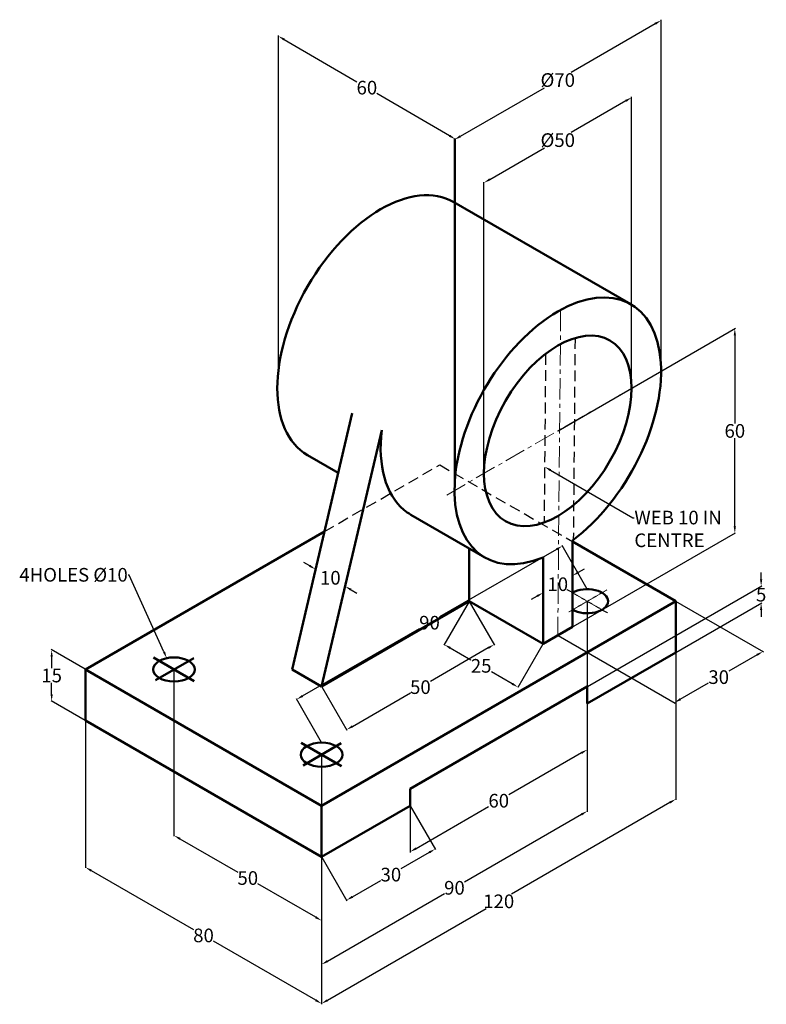
# Model space of a CAD drawing. Units: millimetres. Extents: x -58 to 161, y -39 to 250.
import ezdxf
from ezdxf import colors
from ezdxf.entities.mleader import LeaderData, LeaderLine
from ezdxf.math import Vec2, Vec3

# ---------------------------------------------------------------- set-up
doc = ezdxf.new("R2010")
doc.units = ezdxf.units.MM
doc.header["$MEASUREMENT"] = 0
doc.linetypes.add('CENTER', pattern=[2, 1.25, -0.25, 0.25, -0.25])
doc.linetypes.add('HIDDEN', pattern=[9.525, 6.35, -3.175])
for name, color, linetype, lineweight in [('M-CNTR', 1, 'CENTER', 18), ('M-DIMS', 2, 'Continuous', 25), ('M-HIDN', 3, 'HIDDEN', 25), ('M-OUTL', 7, 'Continuous', 50)]:
    doc.layers.add(name, color=color, linetype=linetype, lineweight=lineweight)
doc.styles.get("Standard").update_dxf_attribs({"font": 'arial.ttf'})
doc.dimstyles.get("Standard").update_dxf_attribs({"dimtxt": 4, "dimasz": 2, "dimexe": 0.18, "dimexo": 0.0625, "dimgap": 0.09, "dimtad": 0, "dimtih": 1, "dimtoh": 1, "dimdec": 0, "dimzin": 0, "dimdsep": 46, "dimtxsty": 'Standard', "dimcen": 0.09, "dimadec": 0, "dimazin": 0, "dimtfac": 1, "dimtdec": 0, "dimtofl": 0, "dimtmove": 0, "dimatfit": 3, "dimfxl": 1, "dimtolj": 1, "dimtzin": 0, "dimarcsym": 0})

# ---------------------------------------------------------------- blocks, each defined once
blk = doc.blocks.new('*D1')
at = {"layer": 'Defpoints', "color": 0, "transparency": 16777216}
for p in [(-12.58, 59.39), (30.72, 34.39), (-12.58, 10.7)]:
    blk.add_point(p, dxfattribs=at)
at = {"layer": 'M-DIMS', "color": 0, "lineweight": -2, "transparency": 16777216}
for p, q in [((-12.58, 59.32), (-12.58, 10.49)), ((30.72, 34.32), (30.72, -14.51)), ((-10.85, 9.7), (6.12, -0.1)), ((28.99, -13.3), (12.02, -3.5))]:
    blk.add_line(p, q, dxfattribs=at)
at = {"layer": 'M-DIMS', "color": 0, "transparency": 16777216}
for points in [[(-10.68, 9.99), (-11.01, 9.41), (-12.58, 10.7)], [(29.16, -13.01), (28.82, -13.59), (30.72, -14.3)]]:
    blk.add_solid(points, dxfattribs=at)
at = {"layer": 'M-DIMS', "color": 0, "transparency": 16777216, "insert": (9.07, -1.8), "char_height": 4, "attachment_point": 5}
blk.add_mtext('\\A1;50', dxfattribs=at)
blk = doc.blocks.new('*D2')
at = {"layer": 'Defpoints', "color": 0, "transparency": 16777216}
for p in [(-38.56, 44.39), (30.72, 4.39), (-38.56, 1.36)]:
    blk.add_point(p, dxfattribs=at)
at = {"layer": 'M-DIMS', "color": 0, "lineweight": -2, "transparency": 16777216}
for p, q in [((-38.56, 44.32), (-38.56, 1.15)), ((30.72, 4.32), (30.72, -38.85)), ((-36.83, 0.36), (-6.87, -16.94)), ((28.99, -37.64), (-0.97, -20.34))]:
    blk.add_line(p, q, dxfattribs=at)
at = {"layer": 'M-DIMS', "color": 0, "transparency": 16777216}
for points in [[(-36.66, 0.65), (-36.99, 0.07), (-38.56, 1.36)], [(29.16, -37.35), (28.82, -37.93), (30.72, -38.64)]]:
    blk.add_solid(points, dxfattribs=at)
at = {"layer": 'M-DIMS', "color": 0, "transparency": 16777216, "insert": (-3.92, -18.64), "char_height": 4, "attachment_point": 5}
blk.add_mtext('\\A1;80', dxfattribs=at)
blk = doc.blocks.new('*D3')
at = {"layer": 'Defpoints', "color": 0, "transparency": 16777216}
for p in [(-48.47, 65.11), (-38.56, 59.39), (-38.56, 44.39)]:
    blk.add_point(p, dxfattribs=at)
at = {"layer": 'M-DIMS', "color": 0, "lineweight": -2, "transparency": 16777216}
for p, q in [((-38.62, 59.43), (-48.65, 65.21)), ((-48.47, 63.11), (-48.47, 59.74)), ((-48.47, 52.11), (-48.47, 55.48)), ((-38.62, 44.43), (-48.65, 50.21))]:
    blk.add_line(p, q, dxfattribs=at)
at = {"layer": 'M-DIMS', "color": 0, "transparency": 16777216}
for points in [[(-48.8, 63.11), (-48.13, 63.11), (-48.47, 65.11)], [(-48.8, 52.11), (-48.13, 52.11), (-48.47, 50.11)]]:
    blk.add_solid(points, dxfattribs=at)
at = {"layer": 'M-DIMS', "color": 0, "transparency": 16777216, "insert": (-48.47, 57.61), "char_height": 4, "attachment_point": 5}
blk.add_mtext('\\A1;15', dxfattribs=at)
blk = doc.blocks.new('*D4')
at = {"layer": 'Defpoints', "color": 0, "transparency": 16777216}
for p in [(108.66, 54.39), (108.66, 35.88), (56.7, 24.39)]:
    blk.add_point(p, dxfattribs=at)
at = {"layer": 'M-DIMS', "color": 0, "lineweight": -2, "transparency": 16777216}
for p, q in [((108.66, 54.32), (108.66, 35.67)), ((106.93, 34.88), (85.64, 22.59)), ((56.7, 24.32), (56.7, 5.67)), ((58.43, 6.88), (79.72, 19.17))]:
    blk.add_line(p, q, dxfattribs=at)
at = {"layer": 'M-DIMS', "color": 0, "transparency": 16777216}
for points in [[(106.77, 35.17), (107.1, 34.59), (108.66, 35.88)], [(58.27, 7.17), (58.6, 6.59), (56.7, 5.88)]]:
    blk.add_solid(points, dxfattribs=at)
at = {"layer": 'M-DIMS', "color": 0, "transparency": 16777216, "insert": (82.68, 20.88), "char_height": 4, "attachment_point": 5}
blk.add_mtext('\\A1;60', dxfattribs=at)
blk = doc.blocks.new('*D5')
at = {"layer": 'Defpoints', "color": 0, "transparency": 16777216}
for p in [(108.66, 79.39), (30.72, 34.39), (108.66, 17.83)]:
    blk.add_point(p, dxfattribs=at)
at = {"layer": 'M-DIMS', "color": 0, "lineweight": -2, "transparency": 16777216}
for p, q in [((108.66, 79.32), (108.66, 17.62)), ((30.72, 34.32), (30.72, -27.38)), ((106.93, 16.83), (72.64, -2.97)), ((32.45, -26.17), (66.74, -6.37))]:
    blk.add_line(p, q, dxfattribs=at)
at = {"layer": 'M-DIMS', "color": 0, "transparency": 16777216}
for points in [[(106.77, 17.12), (107.1, 16.54), (108.66, 17.83)], [(32.29, -25.88), (32.62, -26.46), (30.72, -27.17)]]:
    blk.add_solid(points, dxfattribs=at)
at = {"layer": 'M-DIMS', "color": 0, "transparency": 16777216, "insert": (69.69, -4.67), "char_height": 4, "attachment_point": 5}
blk.add_mtext('\\A1;90', dxfattribs=at)
blk = doc.blocks.new('*D6')
at = {"layer": 'Defpoints', "color": 0, "transparency": 16777216}
for p in [(134.64, 79.39), (134.64, 21.36), (30.72, 19.39)]:
    blk.add_point(p, dxfattribs=at)
at = {"layer": 'M-DIMS', "color": 0, "lineweight": -2, "transparency": 16777216}
for p, q in [((134.64, 79.32), (134.64, 21.15)), ((132.91, 20.36), (86.38, -6.51)), ((30.72, 19.32), (30.72, -38.85)), ((32.45, -37.64), (78.99, -10.77))]:
    blk.add_line(p, q, dxfattribs=at)
at = {"layer": 'M-DIMS', "color": 0, "transparency": 16777216}
for points in [[(132.75, 20.65), (133.08, 20.07), (134.64, 21.36)], [(32.29, -37.35), (32.62, -37.93), (30.72, -38.64)]]:
    blk.add_solid(points, dxfattribs=at)
at = {"layer": 'M-DIMS', "color": 0, "transparency": 16777216, "insert": (82.68, -8.64), "char_height": 4, "attachment_point": 5}
blk.add_mtext('\\A1;120', dxfattribs=at)
blk = doc.blocks.new('*D7')
at = {"layer": 'Defpoints', "color": 0, "transparency": 16777216}
for p in [(125.97, 84.4), (100, 69.39), (160.18, 64.65)]:
    blk.add_point(p, dxfattribs=at)
at = {"layer": 'M-DIMS', "color": 0, "lineweight": -2, "transparency": 16777216}
for p, q in [((126.03, 84.36), (160.36, 64.54)), ((100.07, 69.35), (134.4, 49.53)), ((158.45, 63.65), (150.15, 58.85)), ((135.95, 50.64), (144.25, 55.44))]:
    blk.add_line(p, q, dxfattribs=at)
at = {"layer": 'M-DIMS', "color": 0, "transparency": 16777216}
for points in [[(158.28, 63.94), (158.61, 63.36), (160.18, 64.65)], [(135.78, 50.93), (136.12, 50.35), (134.22, 49.64)]]:
    blk.add_solid(points, dxfattribs=at)
at = {"layer": 'M-DIMS', "color": 0, "transparency": 16777216, "insert": (147.2, 57.14), "char_height": 4, "attachment_point": 5}
blk.add_mtext('\\A1;30', dxfattribs=at)
blk = doc.blocks.new('*D8')
at = {"layer": 'Defpoints', "color": 0, "transparency": 16777216}
for p in [(151.94, 159.37), (100, 129.39), (100, 69.39)]:
    blk.add_point(p, dxfattribs=at)
at = {"layer": 'M-DIMS', "color": 0, "lineweight": -2, "transparency": 16777216}
for p, q in [((100.07, 129.43), (152.12, 159.48)), ((151.94, 157.37), (151.94, 131.5)), ((151.94, 101.37), (151.94, 127.24)), ((100.07, 69.43), (152.12, 99.48))]:
    blk.add_line(p, q, dxfattribs=at)
at = {"layer": 'M-DIMS', "color": 0, "transparency": 16777216}
for points in [[(151.6, 157.37), (152.27, 157.37), (151.94, 159.37)], [(151.6, 101.37), (152.27, 101.37), (151.94, 99.37)]]:
    blk.add_solid(points, dxfattribs=at)
at = {"layer": 'M-DIMS', "color": 0, "transparency": 16777216, "insert": (151.94, 129.37), "char_height": 4, "attachment_point": 5}
blk.add_mtext('\\A1;60', dxfattribs=at)
blk = doc.blocks.new('*D9')
at = {"layer": 'Defpoints', "color": 0, "transparency": 16777216}
for p in [(95.67, 81.9), (104.33, 71.89), (95.67, 66.89)]:
    blk.add_point(p, dxfattribs=at)
at = {"layer": 'M-DIMS', "color": 0, "lineweight": -2, "transparency": 16777216}
for p, q in [((104.33, 71.96), (104.33, 87.1)), ((106.07, 87.9), (107.8, 88.9)), ((93.94, 80.9), (92.21, 79.9)), ((95.67, 66.96), (95.67, 82.1))]:
    blk.add_line(p, q, dxfattribs=at)
at = {"layer": 'M-DIMS', "color": 0, "transparency": 16777216}
for points in [[(105.9, 88.18), (106.23, 87.61), (104.33, 86.9)], [(93.78, 81.18), (94.11, 80.61), (95.67, 81.9)]]:
    blk.add_solid(points, dxfattribs=at)
at = {"layer": 'M-DIMS', "color": 0, "transparency": 16777216, "insert": (100, 84.4), "char_height": 4, "attachment_point": 5}
blk.add_mtext('\\A1;10', dxfattribs=at)
blk = doc.blocks.new('*D10')
at = {"layer": 'Defpoints', "color": 0, "transparency": 16777216}
for p in [(37.61, 83.78), (22.06, 59.39), (30.72, 54.39)]:
    blk.add_point(p, dxfattribs=at)
at = {"layer": 'M-DIMS', "color": 0, "lineweight": -2, "transparency": 16777216}
for p, q in [((27.22, 89.78), (25.49, 90.78)), ((22.08, 59.45), (29, 88.96)), ((30.74, 54.45), (37.66, 83.96)), ((39.35, 82.78), (41.08, 81.78))]:
    blk.add_line(p, q, dxfattribs=at)
at = {"layer": 'M-DIMS', "color": 0, "transparency": 16777216}
for points in [[(27.39, 90.07), (27.06, 89.49), (28.95, 88.78)], [(39.51, 83.07), (39.18, 82.49), (37.61, 83.78)]]:
    blk.add_solid(points, dxfattribs=at)
at = {"layer": 'M-DIMS', "color": 0, "transparency": 16777216, "insert": (33.28, 86.28), "char_height": 4, "attachment_point": 5}
blk.add_mtext('\\A1;10', dxfattribs=at)
blk = doc.blocks.new('*D11')
at = {"layer": 'Defpoints', "color": 0, "transparency": 16777216}
for p in [(18.03, 245.2), (18.03, 146.96), (69.97, 116.73)]:
    blk.add_point(p, dxfattribs=at)
at = {"layer": 'M-DIMS', "color": 0, "lineweight": -2, "transparency": 16777216}
for p, q in [((18.03, 147.03), (18.03, 245.4)), ((19.76, 244.19), (41.04, 231.8)), ((68.24, 215.97), (46.96, 228.36)), ((69.97, 116.8), (69.97, 215.17))]:
    blk.add_line(p, q, dxfattribs=at)
at = {"layer": 'M-DIMS', "color": 0, "transparency": 16777216}
for points in [[(19.93, 244.48), (19.59, 243.9), (18.03, 245.2)], [(68.4, 216.26), (68.07, 215.68), (69.97, 214.97)]]:
    blk.add_solid(points, dxfattribs=at)
at = {"layer": 'M-DIMS', "color": 0, "transparency": 16777216, "insert": (44, 230.08), "char_height": 4, "attachment_point": 5}
blk.add_mtext('\\A1;60', dxfattribs=at)
blk = doc.blocks.new('*D12')
at = {"layer": 'Defpoints', "color": 0, "transparency": 16777216}
for p in [(121.65, 227.18), (121.65, 141.89), (78.35, 116.89)]:
    blk.add_point(p, dxfattribs=at)
at = {"layer": 'M-DIMS', "color": 0, "lineweight": -2, "transparency": 16777216}
for p, q in [((119.92, 226.18), (103.89, 216.93)), ((121.65, 141.96), (121.65, 227.39)), ((80.09, 203.18), (96.12, 212.44)), ((78.35, 116.96), (78.35, 202.39))]:
    blk.add_line(p, q, dxfattribs=at)
at = {"layer": 'M-DIMS', "color": 0, "transparency": 16777216}
for points in [[(119.76, 226.47), (120.09, 225.89), (121.65, 227.18)], [(79.92, 203.47), (80.25, 202.89), (78.35, 202.18)]]:
    blk.add_solid(points, dxfattribs=at)
at = {"layer": 'M-DIMS', "color": 0, "transparency": 16777216, "insert": (100, 214.68), "char_height": 4, "attachment_point": 5}
blk.add_mtext('\\A1;%%C50', dxfattribs=at)
blk = doc.blocks.new('*D13')
at = {"layer": 'Defpoints', "color": 0, "transparency": 16777216}
for p in [(130.31, 249.81), (130.31, 146.89), (69.69, 111.89)]:
    blk.add_point(p, dxfattribs=at)
at = {"layer": 'M-DIMS', "color": 0, "lineweight": -2, "transparency": 16777216}
for p, q in [((128.58, 248.81), (103.89, 234.55)), ((130.31, 146.96), (130.31, 250.02)), ((71.43, 215.81), (96.12, 230.06)), ((69.69, 111.96), (69.69, 215.02))]:
    blk.add_line(p, q, dxfattribs=at)
at = {"layer": 'M-DIMS', "color": 0, "transparency": 16777216}
for points in [[(128.42, 249.1), (128.75, 248.52), (130.31, 249.81)], [(71.26, 216.1), (71.59, 215.52), (69.69, 214.81)]]:
    blk.add_solid(points, dxfattribs=at)
at = {"layer": 'M-DIMS', "color": 0, "transparency": 16777216, "insert": (100, 232.31), "char_height": 4, "attachment_point": 5}
blk.add_mtext('\\A1;%%C70', dxfattribs=at)
blk = doc.blocks.new('*D14')
at = {"layer": 'Defpoints', "color": 0, "transparency": 16777216}
for p in [(159.66, 78.83), (108.66, 54.39), (108.66, 49.39)]:
    blk.add_point(p, dxfattribs=at)
at = {"layer": 'M-DIMS', "color": 0, "lineweight": -2, "transparency": 16777216}
for p, q in [((159.66, 85.83), (159.66, 87.83)), ((108.73, 54.43), (159.84, 83.93)), ((108.73, 49.43), (159.84, 78.93)), ((159.66, 76.83), (159.66, 74.83))]:
    blk.add_line(p, q, dxfattribs=at)
at = {"layer": 'M-DIMS', "color": 0, "transparency": 16777216}
for points in [[(159.32, 85.83), (159.99, 85.83), (159.66, 83.83)], [(159.32, 76.83), (159.99, 76.83), (159.66, 78.83)]]:
    blk.add_solid(points, dxfattribs=at)
at = {"layer": 'M-DIMS', "color": 0, "transparency": 16777216, "insert": (159.66, 81.33), "char_height": 4, "attachment_point": 5}
blk.add_mtext('\\A1;5', dxfattribs=at)
blk = doc.blocks.new('HOLE-ISO')
at = {"ltscale": 0.1}
for p, q in [((0.13, 7), (11.99, 0.15)), ((0.71, 0.41), (11.9, 6.87))]:
    blk.add_line(p, q, dxfattribs=at)
blk.add_ellipse((6.12, 3.54), major_axis=(-6.12, 0), ratio=0.57735)
blk = doc.blocks.new('*D16')
at = {"layer": 'Defpoints', "color": 0, "transparency": 16777216}
for p in [(56.7, 19.39), (30.72, 4.39), (38.05, -8.3)]:
    blk.add_point(p, dxfattribs=at)
at = {"layer": 'M-DIMS', "color": 0, "lineweight": -2, "transparency": 16777216}
for p, q in [((56.73, 19.34), (64.12, 6.55)), ((30.75, 4.34), (38.14, -8.45)), ((62.3, 5.7), (53.98, 0.9)), ((39.78, -7.3), (48.09, -2.5))]:
    blk.add_line(p, q, dxfattribs=at)
at = {"layer": 'M-DIMS', "color": 0, "transparency": 16777216}
for points in [[(62.13, 5.99), (62.46, 5.41), (64.03, 6.7)], [(39.61, -7.01), (39.95, -7.59), (38.05, -8.3)]]:
    blk.add_solid(points, dxfattribs=at)
at = {"layer": 'M-DIMS', "color": 0, "transparency": 16777216, "insert": (51.04, -0.8), "char_height": 4, "attachment_point": 5}
blk.add_mtext('\\A1;30', dxfattribs=at)
blk = doc.blocks.new('*D17')
at = {"layer": 'Defpoints', "color": 0, "transparency": 16777216}
for p in [(74.02, 79.39), (30.72, 54.39), (38.05, 41.7)]:
    blk.add_point(p, dxfattribs=at)
at = {"layer": 'M-DIMS', "color": 0, "lineweight": -2, "transparency": 16777216}
for p, q in [((74.05, 79.34), (81.44, 66.55)), ((79.62, 65.7), (62.65, 55.9)), ((30.75, 54.34), (38.14, 41.55)), ((39.78, 42.7), (56.75, 52.5))]:
    blk.add_line(p, q, dxfattribs=at)
at = {"layer": 'M-DIMS', "color": 0, "transparency": 16777216}
for points in [[(79.45, 65.99), (79.78, 65.41), (81.35, 66.7)], [(39.61, 42.99), (39.95, 42.41), (38.05, 41.7)]]:
    blk.add_solid(points, dxfattribs=at)
at = {"layer": 'M-DIMS', "color": 0, "transparency": 16777216, "insert": (59.7, 54.2), "char_height": 4, "attachment_point": 5}
blk.add_mtext('\\A1;50', dxfattribs=at)
blk = doc.blocks.new('*D18')
at = {"layer": 'Defpoints', "color": 0, "transparency": 16777216}
for p in [(74.02, 79.39), (66.7, 66.7), (95.67, 66.89)]:
    blk.add_point(p, dxfattribs=at)
at = {"layer": 'M-DIMS', "color": 0, "lineweight": -2, "transparency": 16777216}
for p, q in [((73.99, 79.34), (66.61, 66.55)), ((95.64, 66.84), (88.26, 54.05)), ((68.43, 65.7), (74.52, 62.19)), ((86.62, 55.2), (80.53, 58.72))]:
    blk.add_line(p, q, dxfattribs=at)
at = {"layer": 'M-DIMS', "color": 0, "transparency": 16777216}
for points in [[(68.6, 65.99), (68.26, 65.41), (66.7, 66.7)], [(86.78, 55.49), (86.45, 54.91), (88.35, 54.2)]]:
    blk.add_solid(points, dxfattribs=at)
at = {"layer": 'M-DIMS', "color": 0, "transparency": 16777216, "insert": (77.52, 60.45), "char_height": 4, "attachment_point": 5}
blk.add_mtext('\\A1;25', dxfattribs=at)
blk = doc.blocks.new('*D19')
at = {"layer": 'Defpoints', "color": 0, "transparency": 16777216}
for p in [(101.34, 95.61), (108.66, 82.93), (30.72, 37.93)]:
    blk.add_point(p, dxfattribs=at)
at = {"layer": 'M-DIMS', "color": 0, "lineweight": -2, "transparency": 16777216}
for p, q in [((108.63, 82.98), (101.25, 95.77)), ((99.61, 94.61), (65.32, 74.81)), ((25.13, 51.61), (59.42, 71.41)), ((30.69, 37.98), (23.31, 50.77))]:
    blk.add_line(p, q, dxfattribs=at)
at = {"layer": 'M-DIMS', "color": 0, "transparency": 16777216}
for points in [[(99.44, 94.9), (99.77, 94.32), (101.34, 95.61)], [(24.96, 51.9), (25.3, 51.32), (23.4, 50.61)]]:
    blk.add_solid(points, dxfattribs=at)
at = {"layer": 'M-DIMS', "color": 0, "transparency": 16777216, "insert": (62.37, 73.11), "char_height": 4, "attachment_point": 5}
blk.add_mtext('\\A1;90', dxfattribs=at)

msp = doc.modelspace()

# ---------------------------------------------------------------- linework, layer by layer
at = {"layer": 'M-CNTR', "ltscale": 5}
for p, q in [((100.84, 164.86), (100, 69.39)), ((67.41, 110.57), (134.36, 149.22))]:
    msp.add_line(p, q, dxfattribs=at)
at = {"layer": 'M-CNTR', "ltscale": 0.1}
for p, q in [((102.67, 82.85), (114.54, 76)), ((103.25, 76.26), (114.44, 82.73))]:
    msp.add_line(p, q, dxfattribs=at)
at = {"layer": 'M-HIDN', "ltscale": 0.5}
for p, q in [((105.08, 156.62), (104.56, 97.42)), ((96.42, 151.98), (95.99, 102.5)), ((31.56, 99.87), (65.36, 119.39)), ((65.36, 119.39), (104.33, 96.89))]:
    msp.add_line(p, q, dxfattribs=at)
at = {"layer": 'M-OUTL'}
for p, q in [((69.48, 196.51), (121.44, 166.51)), ((39.69, 134.57), (22.06, 59.39)), ((48.35, 129.57), (30.72, 54.39)), ((26.61, 122.27), (35.59, 117.08)), ((56.92, 104.77), (78.57, 92.27)), ((-38.56, 59.39), (31.56, 99.87)), ((104.33, 71.89), (104.33, 97.25)), ((104.33, 96.89), (134.64, 79.39)), ((74.02, 79.39), (74.02, 94.89)), ((95.67, 66.89), (95.67, 92.25)), ((30.72, 19.39), (134.64, 79.39)), ((30.72, 54.39), (74.02, 79.39)), ((74.02, 79.39), (95.67, 66.89)), ((134.64, 79.39), (134.64, 64.39)), ((104.33, 71.89), (95.67, 66.89)), ((134.64, 64.39), (108.66, 49.39)), ((-38.56, 44.39), (-38.56, 59.39)), ((-38.56, 59.39), (30.72, 19.39)), ((22.06, 59.39), (30.72, 54.39)), ((26.39, 56.89), (22.06, 59.39)), ((22.06, 59.39), (30.72, 54.39)), ((108.66, 54.39), (56.7, 24.39)), ((108.66, 49.39), (108.66, 54.39)), ((30.72, 4.39), (-38.56, 44.39)), ((56.7, 24.39), (56.7, 19.39)), ((30.72, 19.39), (30.72, 4.39)), ((56.7, 19.39), (30.72, 4.39))]:
    msp.add_line(p, q, dxfattribs=at)
for centre, major_axis, start_param, end_param in [((48.04, 159.39), (-21.43, -37.12), 3.141593, 6.283185), ((100, 129.39), (-21.43, -37.12), 0.928746, 6.925236), ((78.35, 141.89), (-21.43, -37.12), 5.35444, 6.181997), ((78.35, 141.89), (-21.43, -37.12), 6.181997, 6.283185), ((108.66, 79.39), (-6.12, 0), 0.785398, 5.497787)]:
    msp.add_ellipse(centre, major_axis=major_axis, ratio=0.57735, start_param=start_param, end_param=end_param, dxfattribs=at)
msp.add_ellipse((100, 129.39), major_axis=(-15.31, -26.52), ratio=0.57735, dxfattribs=at)

# ---------------------------------------------------------------- block references
for p in [(-18.7, 55.85), (24.6, 30.85)]:
    msp.add_blockref('HOLE-ISO', p, dxfattribs=at)

# ---------------------------------------------------------------- dimensions: what is measured, and where the dimension line sits
at = {"layer": 'M-DIMS'}
dim = msp.add_aligned_dim(p1=(69.69, 111.89), p2=(130.31, 146.89), distance=89.13, text='%%C<>', dimstyle='Standard', override={"dimclrd": 0, "dimclre": 0, "dimclrt": 0}, dxfattribs=at)
dim.commit()
dim.dimension.update_dxf_attribs({"geometry": '*D13', "text_midpoint": (100, 232.31)})
for p1, p2, distance, picture, middle in [((69.97, 116.73), (18.03, 146.96), -84.9, '*D11', (44, 230.08)), ((100, 69.39), (100, 129.39), -51.93, '*D8', (151.94, 129.37)), ((22.06, 59.39), (30.72, 54.39), 28.9, '*D10', (33.28, 86.28)), ((104.33, 71.89), (95.67, 66.89), -13, '*D9', (100, 84.4)), ((108.66, 54.39), (108.66, 49.39), 50.99, '*D14', (159.66, 81.33)), ((100, 69.39), (125.97, 84.4), -34.23, '*D7', (147.2, 57.14)), ((30.72, 34.39), (108.66, 79.39), -53.31, '*D5', (69.69, -4.67)), ((30.72, 19.39), (134.64, 79.39), -50.26, '*D6', (82.68, -8.64)), ((-38.56, 44.39), (-38.56, 59.39), 9.91, '*D3', (-48.47, 57.61)), ((30.72, 34.39), (-12.58, 59.39), 42.17, '*D1', (9.07, -1.8)), ((56.7, 24.39), (108.66, 54.39), -16.03, '*D4', (82.68, 20.88)), ((30.72, 4.39), (-38.56, 44.39), 37.27, '*D2', (-3.92, -18.64))]:
    dim = msp.add_aligned_dim(p1=p1, p2=p2, distance=distance, dimstyle='Standard', override={"dimclrd": 0, "dimclre": 0, "dimclrt": 0}, dxfattribs=at)
    dim.commit()
    dim.dimension.update_dxf_attribs({"geometry": picture, "text_midpoint": middle})
dim = msp.add_linear_dim(base=(121.65, 227.18), p1=(78.35, 116.89), p2=(121.65, 141.89), angle=30, text='%%C<>', dimstyle='Standard', override={"dimclrd": 0, "dimclre": 0, "dimclrt": 0}, dxfattribs=at)
dim.commit()
dim.dimension.update_dxf_attribs({"geometry": '*D12', "text_midpoint": (100, 214.68), "dimtype": 161})
for base, p1, p2, angle, picture, middle in [((101.34, 95.61), (30.72, 37.93), (108.66, 82.93), 30, '*D19', (62.37, 73.11)), ((38.05, 41.7), (74.02, 79.39), (30.72, 54.39), 210, '*D17', (59.7, 54.2)), ((66.7, 66.7), (95.67, 66.89), (74.02, 79.39), 150, '*D18', (77.52, 60.45)), ((38.05, -8.3), (56.7, 19.39), (30.72, 4.39), 210, '*D16', (51.04, -0.8))]:
    dim = msp.add_linear_dim(base=base, p1=p1, p2=p2, angle=angle, dimstyle='Standard', override={"dimdec": 0, "dimlfac": 1, "dimrnd": 0, "dimzin": 0, "dimdsep": 46, "dimlunit": 2}, dxfattribs=at)
    dim.commit()
    dim.dimension.update_dxf_attribs({"geometry": picture, "text_midpoint": middle})

# ---------------------------------------------------------------- leaders
ml = msp.add_multileader_mtext('Standard', dxfattribs=at)
ml.set_content('WEB 10 IN\\PCENTRE', color=256)
ml.set_leader_properties()
ml.build(insert=Vec2(0, 0))
ml.multileader.update_dxf_attribs({"dogleg_length": 0.36, "arrow_head_size": 2})
ctx = ml.context
ctx.base_point, ctx.arrow_head_size, ctx.landing_gap_size, ctx.plane_origin = Vec3(122.38, 103.91), 2, 0.09, Vec3(96.13, 118.86)
notes = []
notes.append((ctx, [(0, (1, 1, 0), (122.02, 103.91), (1, 0), 0.36, [(0, [(96.13, 118.86)], 0, [])])]))
ctx.mtext.insert, ctx.mtext.flow_direction = Vec3(122.47, 105.95), 5
ml = msp.add_multileader_mtext('Standard', dxfattribs=at)
ml.set_content('4HOLES %%C10', color=256)
ml.set_leader_properties()
ml.build(insert=Vec2(0, 0))
ml.multileader.update_dxf_attribs({"dogleg_length": 0.36, "arrow_head_size": 2})
ctx = ml.context
ctx.base_point, ctx.arrow_head_size, ctx.landing_gap_size, ctx.plane_origin = Vec3(-60.06, 87.08), 2, 0.09, Vec3(-14.7, 62.71)
ctx.text_align_type = 2
notes.append((ctx, [(0, (1, 1, 0), (-25.69, 87.08), (-1, 0), 0.36, [(0, [(-14.7, 62.71)], 0, [])])]))
ctx.mtext.insert, ctx.mtext.alignment, ctx.mtext.flow_direction = Vec3(-26.14, 89.16), 3, 5
for ctx, leaders in notes:
    for number, flags, end, landing, length, lines in leaders:
        leader = LeaderData()
        leader.index, (leader.has_last_leader_line, leader.has_dogleg_vector, leader.attachment_direction) = number, flags
        leader.last_leader_point, leader.dogleg_vector, leader.dogleg_length = Vec3(end), Vec3(landing), length
        for number, points, colour, breaks in lines:
            line = LeaderLine()
            line.index, line.vertices, line.color, line.breaks = number, Vec3.list(points), colors.encode_raw_color(colour), breaks
            leader.lines.append(line)
        ctx.leaders.append(leader)

doc.saveas('drawing.dxf')
